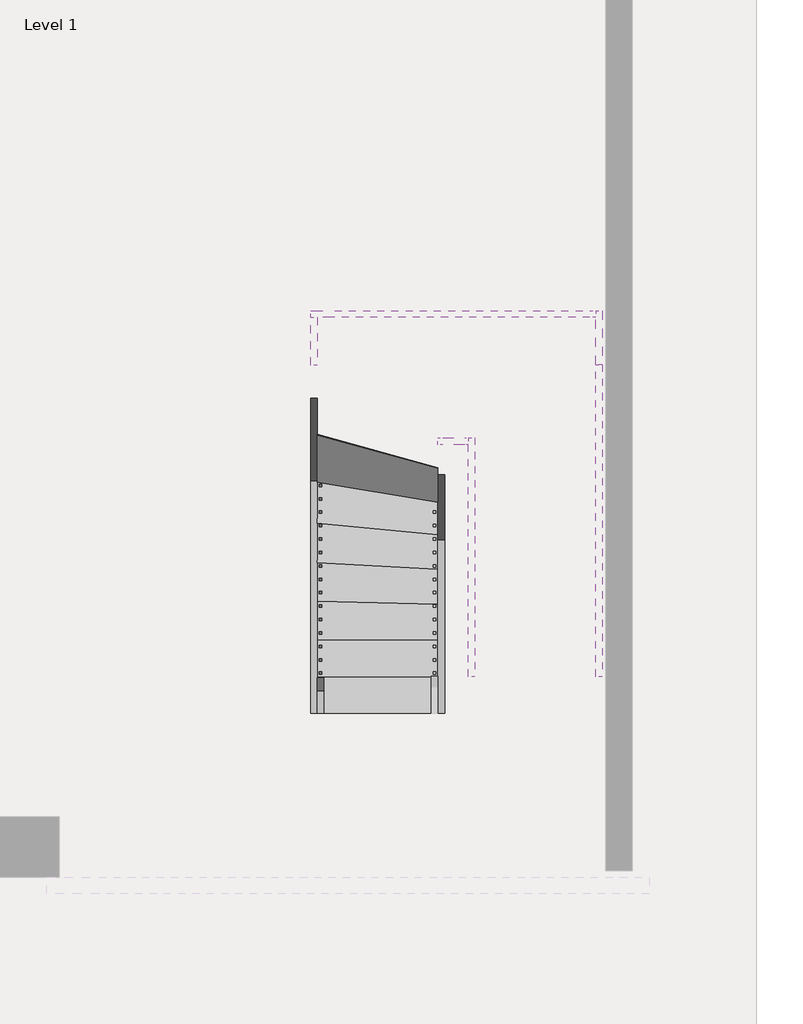
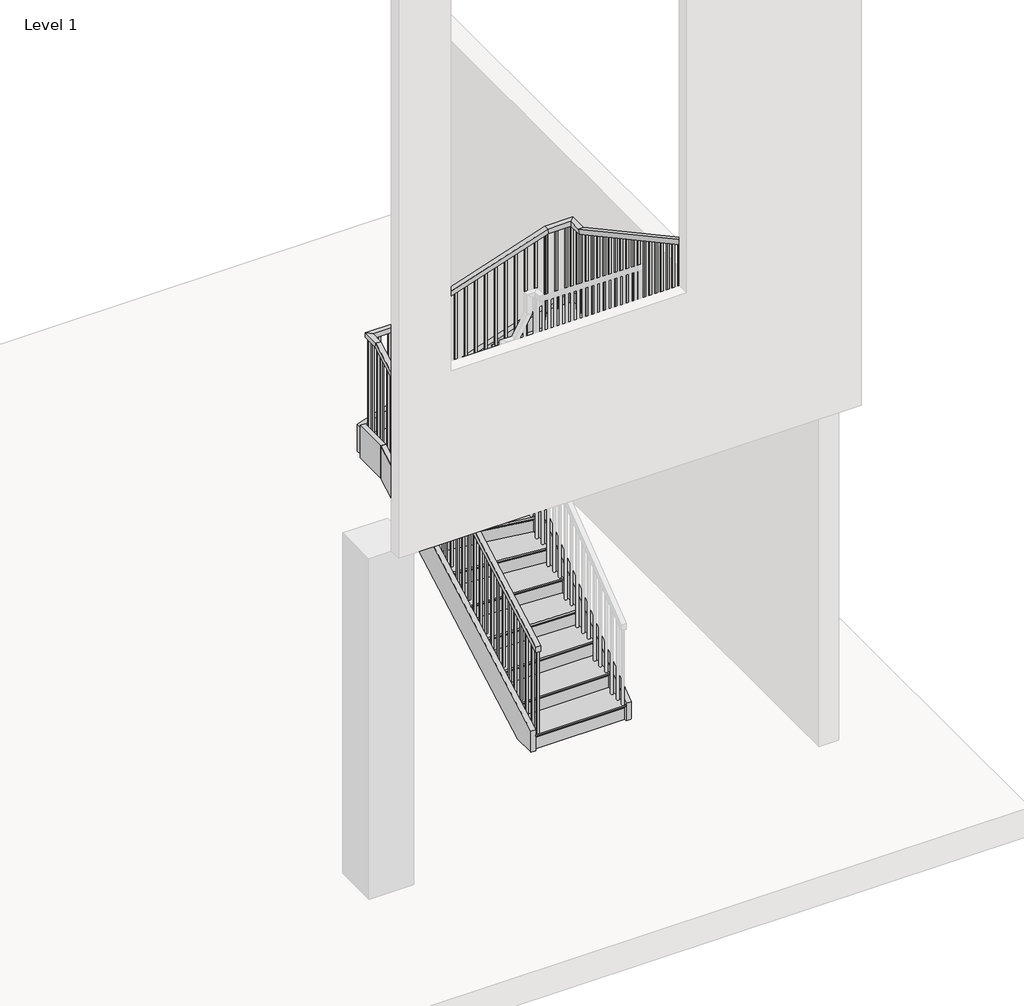
# One storey, part 2 of 2: 8 members, 1 railing, 1 stair flight.
"""IFC4 building model written with IfcOpenShell, lengths in millimetres."""

from ifc_helpers import new_model, si_unit, frame, origin, place, context, project, spatial, polyline, outline, extrude, faceted_brep, transform, mapped, element, save
from components import stair_flight_cb62f9a1

model = new_model("IFC4")

# Units and contexts
model_context = context("Model", 3, world=origin())
ifc_project = project(units=[si_unit("LENGTHUNIT", "METRE", prefix="MILLI")], contexts=[model_context])

# Site, building, storey
site = spatial("IfcSite", under=ifc_project)
building = spatial("IfcBuilding", under=site)
storey = spatial("IfcBuildingStorey", under=building, Name="Level 1", Elevation=0.0)

# Members
placement = place(None, origin())
element("IfcMember", 1, ObjectType="Stringer - 2\" Width", at=placement, inside=storey, context=model_context, shape_type="SweptSolid", body=[
    extrude(outline(polyline([(6052.3300735, 0.0), (6052.3300735, 226.8967502), (8691.4859641, 1688.3473575), (8691.4859641, 1339.9346078), (6271.7693513, 0.0), (6052.3300735, 0.0)])), frame((-8157.032922, 0.0, 0.0), z_axis=(1.0, 0.0, 0.0), x_axis=(0.0, 1.0, 0.0)), (0.0, 0.0, 1.0), 50.8),
])
element("IfcMember", 2, ObjectType="Stringer - 2\" Width", at=placement, inside=storey, context=model_context, shape_type="SweptSolid", body=[
    extrude(outline(polyline([(-8106.232922, 8691.4859641), (-8157.032922, 8691.4859641), (-8157.032922, 9053.2617654), (-8106.232922, 9053.2617654), (-8106.232922, 8691.4859641)])), frame((0.0, 0.0, 1339.9346078), z_axis=(0.0, 0.0, 1.0), x_axis=(1.0, 0.0, 0.0)), (0.0, 0.0, 1.0), 348.4127497),
])
element("IfcMember", 3, ObjectType="Stringer - 2\" Width", at=placement, inside=storey, context=model_context, shape_type="SweptSolid", body=[
    extrude(outline(polyline([(1671.581207, -8157.032922), (1383.5473575, -8157.032922), (1383.5473575, -7974.0900261), (2035.7298543, -5998.032922), (2369.5213068, -5998.032922), (2369.5213068, -6042.3341999), (1671.581207, -8157.032922)])), frame((0.0, 9053.2617654, 0.0), z_axis=(0.0, 1.0, 0.0), x_axis=(0.0, 0.0, 1.0)), (0.0, 0.0, 1.0), 50.8),
])
element("IfcMember", 4, ObjectType="Stringer - 2\" Width", at=placement, inside=storey, context=model_context, shape_type="SweptSolid", body=[
    extrude(outline(polyline([(-5998.032922, 9104.0617654), (-5947.232922, 9104.0617654), (-5947.232922, 8694.4281729), (-5998.032922, 8694.4281729), (-5998.032922, 9104.0617654)])), frame((0.0, 0.0, 2048.5496929), z_axis=(0.0, 0.0, 1.0), x_axis=(1.0, 0.0, 0.0)), (0.0, 0.0, 1.0), 320.9716139),
])
element("IfcMember", 5, ObjectType="Stringer - 2\" Width", at=placement, inside=storey, context=model_context, shape_type="SweptSolid", body=[
    extrude(outline(polyline([(8694.4281729, 2369.5213068), (8694.4281729, 2048.5496929), (6331.7300735, 3333.0016037), (6331.7300735, 3653.9732176), (8694.4281729, 2369.5213068)])), frame((-5998.032922, 0.0, 0.0), z_axis=(1.0, 0.0, 0.0), x_axis=(0.0, 1.0, 0.0)), (0.0, 0.0, 1.0), 50.8),
])
element("IfcMember", 6, ObjectType="Stringer - 2\" Width", at=placement, inside=storey, context=model_context, shape_type="SweptSolid", body=[
    extrude(outline(polyline([(6052.3300735, 0.0), (6052.3300735, 188.0018686), (8088.0617654, 1759.6054409), (8088.0617654, 1374.5429999), (6307.5868441, 0.0), (6052.3300735, 0.0)])), frame((-7191.832922, 0.0, 0.0), z_axis=(1.0, 0.0, 0.0), x_axis=(0.0, 1.0, 0.0)), (0.0, 0.0, 1.0), 50.8),
])
element("IfcMember", 7, ObjectType="Stringer - 2\" Width", at=placement, inside=storey, context=model_context, shape_type="SweptSolid", body=[
    extrude(outline(polyline([(1964.5655705, -7191.832922), (1413.7610667, -7191.832922), (1413.7610667, -7154.6813178), (1750.0370706, -6963.232922), (2320.9680273, -6963.232922), (2320.9680273, -6988.9261496), (1964.5655705, -7191.832922)])), frame((0.0, 8088.0617654, 0.0), z_axis=(0.0, 1.0, 0.0), x_axis=(0.0, 0.0, 1.0)), (0.0, 0.0, 1.0), 50.8),
])
element("IfcMember", 8, ObjectType="Stringer - 2\" Width", at=placement, inside=storey, context=model_context, shape_type="SweptSolid", body=[
    extrude(outline(polyline([(8138.8617654, 2320.9680273), (8138.8617654, 1930.7796979), (6331.7300735, 3375.0977978), (6331.7300735, 3765.2861272), (8138.8617654, 2320.9680273)])), frame((-6963.232922, 0.0, 0.0), z_axis=(1.0, 0.0, 0.0), x_axis=(0.0, 1.0, 0.0)), (0.0, 0.0, 1.0), 50.8),
])

# Railing
element("IfcRailing", 9, ObjectType="Handrail - Rectangular", at=placement, inside=storey, context=model_context, shape_type="SolidModel", body=[
    faceted_brep([(-8106.232922, 6052.3300735, 1108.0231981), (-8106.232922, 6052.3300735, 1049.9544064), (-8055.432922, 6052.3300735, 1049.9544064), (-8055.432922, 6052.3300735, 1108.0231981), (-8106.232922, 8867.2431395, 2666.8005421), (-8106.232922, 8880.3694635, 2616.0005421), (-8055.432922, 8880.3694635, 2616.0005421), (-8055.432922, 8867.2431395, 2666.8005421), (-8106.232922, 9053.2617654, 2666.8005421), (-8106.232922, 9053.2617654, 2616.0005421), (-8055.432922, 9002.4617654, 2616.0005421), (-8055.432922, 9002.4617654, 2666.8005421), (-7811.3412458, 9053.2617654, 2666.8005421), (-7803.1748117, 9053.2617654, 2616.0005421), (-7803.1748117, 9002.4617654, 2616.0005421), (-7811.3412458, 9002.4617654, 2666.8005421), (-6285.3448041, 9053.2617654, 3170.4439679), (-6277.17837, 9053.2617654, 3119.6439679), (-6277.17837, 9002.4617654, 3119.6439679), (-6285.3448041, 9002.4617654, 3170.4439679), (-5998.032922, 9053.2617654, 3170.4439679), (-5998.032922, 9053.2617654, 3119.6439679), (-6048.832922, 9002.4617654, 3119.6439679), (-6048.832922, 9002.4617654, 3170.4439679), (-5998.032922, 8868.8551356, 3170.4439679), (-5998.032922, 8855.9393392, 3119.6439679), (-6048.832922, 8855.9393392, 3119.6439679), (-6048.832922, 8868.8551356, 3170.4439679), (-5998.032922, 6331.7300735, 4549.7209626), (-6048.832922, 6331.7300735, 4549.7209626), (-6048.832922, 6331.7300735, 4491.8994479), (-5998.032922, 6331.7300735, 4491.8994479)], [[[0, 1, 2, 3]], [[1, 0, 4, 5]], [[2, 1, 5, 6]], [[3, 2, 6, 7]], [[0, 3, 7, 4]], [[5, 4, 8, 9]], [[6, 5, 9, 10]], [[7, 6, 10, 11]], [[4, 7, 11, 8]], [[9, 8, 12, 13]], [[10, 9, 13, 14]], [[11, 10, 14, 15]], [[8, 11, 15, 12]], [[13, 12, 16, 17]], [[14, 13, 17, 18]], [[15, 14, 18, 19]], [[12, 15, 19, 16]], [[17, 16, 20, 21]], [[18, 17, 21, 22]], [[19, 18, 22, 23]], [[16, 19, 23, 20]], [[21, 20, 24, 25]], [[22, 21, 25, 26]], [[23, 22, 26, 27]], [[20, 23, 27, 24]], [[28, 29, 30, 31]], [[25, 24, 28, 31]], [[26, 25, 31, 30]], [[27, 26, 30, 29]], [[24, 27, 29, 28]]]),
    extrude(outline(polyline([(6439.9801356, 4433.0506263), (6439.9801356, 3483.4285714), (6420.9301356, 3483.4285714), (6420.9301356, 4443.4069257), (6439.9801356, 4433.0506263)])), frame((-6032.957922, 0.0, 0.0), z_axis=(1.0, 0.0, 0.0), x_axis=(0.0, 1.0, 0.0)), (0.0, 0.0, 1.0), 19.05),
    extrude(outline(polyline([(6541.5801356, 4377.8170295), (6541.5801356, 3483.4285714), (6522.5301356, 3483.4285714), (6522.5301356, 4388.1733289), (6541.5801356, 4377.8170295)])), frame((-6032.957922, 0.0, 0.0), z_axis=(1.0, 0.0, 0.0), x_axis=(0.0, 1.0, 0.0)), (0.0, 0.0, 1.0), 19.05),
    extrude(outline(polyline([(6643.1801356, 4322.5834327), (6643.1801356, 3309.2571429), (6624.1301356, 3309.2571429), (6624.1301356, 4332.9397321), (6643.1801356, 4322.5834327)])), frame((-6032.957922, 0.0, 0.0), z_axis=(1.0, 0.0, 0.0), x_axis=(0.0, 1.0, 0.0)), (0.0, 0.0, 1.0), 19.05),
    extrude(outline(polyline([(6744.7801356, 4267.349836), (6744.7801356, 3309.2571429), (6725.7301356, 3309.2571429), (6725.7301356, 4277.7061354), (6744.7801356, 4267.349836)])), frame((-6032.957922, 0.0, 0.0), z_axis=(1.0, 0.0, 0.0), x_axis=(0.0, 1.0, 0.0)), (0.0, 0.0, 1.0), 19.05),
    extrude(outline(polyline([(6846.3801356, 4212.1162392), (6846.3801356, 3309.2571429), (6827.3301356, 3309.2571429), (6827.3301356, 4222.4725386), (6846.3801356, 4212.1162392)])), frame((-6032.957922, 0.0, 0.0), z_axis=(1.0, 0.0, 0.0), x_axis=(0.0, 1.0, 0.0)), (0.0, 0.0, 1.0), 19.05),
    extrude(outline(polyline([(6947.9801356, 4156.8826424), (6947.9801356, 3135.0857143), (6928.9301356, 3135.0857143), (6928.9301356, 4167.2389418), (6947.9801356, 4156.8826424)])), frame((-6032.957922, 0.0, 0.0), z_axis=(1.0, 0.0, 0.0), x_axis=(0.0, 1.0, 0.0)), (0.0, 0.0, 1.0), 19.05),
    extrude(outline(polyline([(7049.5801356, 4101.6490456), (7049.5801356, 3135.0857143), (7030.5301356, 3135.0857143), (7030.5301356, 4112.005345), (7049.5801356, 4101.6490456)])), frame((-6032.957922, 0.0, 0.0), z_axis=(1.0, 0.0, 0.0), x_axis=(0.0, 1.0, 0.0)), (0.0, 0.0, 1.0), 19.05),
    extrude(outline(polyline([(7151.1801356, 4046.4154488), (7151.1801356, 3135.0857143), (7132.1301356, 3135.0857143), (7132.1301356, 4056.7717482), (7151.1801356, 4046.4154488)])), frame((-6032.957922, 0.0, 0.0), z_axis=(1.0, 0.0, 0.0), x_axis=(0.0, 1.0, 0.0)), (0.0, 0.0, 1.0), 19.05),
    extrude(outline(polyline([(7252.7801356, 3991.1818521), (7252.7801356, 2960.9142857), (7233.7301356, 2960.9142857), (7233.7301356, 4001.5381515), (7252.7801356, 3991.1818521)])), frame((-6032.957922, 0.0, 0.0), z_axis=(1.0, 0.0, 0.0), x_axis=(0.0, 1.0, 0.0)), (0.0, 0.0, 1.0), 19.05),
    extrude(outline(polyline([(7354.3801356, 3935.9482553), (7354.3801356, 2960.9142857), (7335.3301356, 2960.9142857), (7335.3301356, 3946.3045547), (7354.3801356, 3935.9482553)])), frame((-6032.957922, 0.0, 0.0), z_axis=(1.0, 0.0, 0.0), x_axis=(0.0, 1.0, 0.0)), (0.0, 0.0, 1.0), 19.05),
    extrude(outline(polyline([(7455.9801356, 3880.7146585), (7455.9801356, 2960.9142857), (7436.9301356, 2960.9142857), (7436.9301356, 3891.0709579), (7455.9801356, 3880.7146585)])), frame((-6032.957922, 0.0, 0.0), z_axis=(1.0, 0.0, 0.0), x_axis=(0.0, 1.0, 0.0)), (0.0, 0.0, 1.0), 19.05),
    extrude(outline(polyline([(7557.5801356, 3825.4810617), (7557.5801356, 2786.7428571), (7538.5301356, 2786.7428571), (7538.5301356, 3835.8373611), (7557.5801356, 3825.4810617)])), frame((-6032.957922, 0.0, 0.0), z_axis=(1.0, 0.0, 0.0), x_axis=(0.0, 1.0, 0.0)), (0.0, 0.0, 1.0), 19.05),
    extrude(outline(polyline([(7659.1801356, 3770.2474649), (7659.1801356, 2786.7428571), (7640.1301356, 2786.7428571), (7640.1301356, 3780.6037643), (7659.1801356, 3770.2474649)])), frame((-6032.957922, 0.0, 0.0), z_axis=(1.0, 0.0, 0.0), x_axis=(0.0, 1.0, 0.0)), (0.0, 0.0, 1.0), 19.05),
    extrude(outline(polyline([(7760.7801356, 3715.0138682), (7760.7801356, 2786.7428571), (7741.7301356, 2786.7428571), (7741.7301356, 3725.3701676), (7760.7801356, 3715.0138682)])), frame((-6032.957922, 0.0, 0.0), z_axis=(1.0, 0.0, 0.0), x_axis=(0.0, 1.0, 0.0)), (0.0, 0.0, 1.0), 19.05),
    extrude(outline(polyline([(7862.3801356, 3659.7802714), (7862.3801356, 2612.5714286), (7843.3301356, 2612.5714286), (7843.3301356, 3670.1365708), (7862.3801356, 3659.7802714)])), frame((-6032.957922, 0.0, 0.0), z_axis=(1.0, 0.0, 0.0), x_axis=(0.0, 1.0, 0.0)), (0.0, 0.0, 1.0), 19.05),
    extrude(outline(polyline([(7963.9801356, 3604.5466746), (7963.9801356, 2612.5714286), (7944.9301356, 2612.5714286), (7944.9301356, 3614.902974), (7963.9801356, 3604.5466746)])), frame((-6032.957922, 0.0, 0.0), z_axis=(1.0, 0.0, 0.0), x_axis=(0.0, 1.0, 0.0)), (0.0, 0.0, 1.0), 19.05),
    extrude(outline(polyline([(8065.5801356, 3549.3130778), (8065.5801356, 2612.5714286), (8046.5301356, 2612.5714286), (8046.5301356, 3559.6693772), (8065.5801356, 3549.3130778)])), frame((-6032.957922, 0.0, 0.0), z_axis=(1.0, 0.0, 0.0), x_axis=(0.0, 1.0, 0.0)), (0.0, 0.0, 1.0), 19.05),
    extrude(outline(polyline([(8167.1801356, 3494.0794811), (8167.1801356, 2438.4), (8148.1301356, 2438.4), (8148.1301356, 3504.4357804), (8167.1801356, 3494.0794811)])), frame((-6032.957922, 0.0, 0.0), z_axis=(1.0, 0.0, 0.0), x_axis=(0.0, 1.0, 0.0)), (0.0, 0.0, 1.0), 19.05),
    extrude(outline(polyline([(8268.7801356, 3438.8458843), (8268.7801356, 2438.4), (8249.7301356, 2438.4), (8249.7301356, 3449.2021837), (8268.7801356, 3438.8458843)])), frame((-6032.957922, 0.0, 0.0), z_axis=(1.0, 0.0, 0.0), x_axis=(0.0, 1.0, 0.0)), (0.0, 0.0, 1.0), 19.05),
    extrude(outline(polyline([(8370.3801356, 3383.6122875), (8370.3801356, 2438.4), (8351.3301356, 2438.4), (8351.3301356, 3393.9685869), (8370.3801356, 3383.6122875)])), frame((-6032.957922, 0.0, 0.0), z_axis=(1.0, 0.0, 0.0), x_axis=(0.0, 1.0, 0.0)), (0.0, 0.0, 1.0), 19.05),
    extrude(outline(polyline([(8471.9801356, 3328.3786907), (8471.9801356, 2438.4), (8452.9301356, 2438.4), (8452.9301356, 3338.7349901), (8471.9801356, 3328.3786907)])), frame((-6032.957922, 0.0, 0.0), z_axis=(1.0, 0.0, 0.0), x_axis=(0.0, 1.0, 0.0)), (0.0, 0.0, 1.0), 19.05),
    extrude(outline(polyline([(8573.5801356, 3273.1450939), (8573.5801356, 2264.2285714), (8554.5301356, 2264.2285714), (8554.5301356, 3283.5013933), (8573.5801356, 3273.1450939)])), frame((-6032.957922, 0.0, 0.0), z_axis=(1.0, 0.0, 0.0), x_axis=(0.0, 1.0, 0.0)), (0.0, 0.0, 1.0), 19.05),
    extrude(outline(polyline([(8675.1801356, 3217.9114972), (8675.1801356, 2264.2285714), (8656.1301356, 2264.2285714), (8656.1301356, 3228.2677965), (8675.1801356, 3217.9114972)])), frame((-6032.957922, 0.0, 0.0), z_axis=(1.0, 0.0, 0.0), x_axis=(0.0, 1.0, 0.0)), (0.0, 0.0, 1.0), 19.05),
    extrude(outline(polyline([(8776.7801356, 3162.6779004), (8776.7801356, 2264.2285714), (8757.7301356, 2264.2285714), (8757.7301356, 3173.0341998), (8776.7801356, 3162.6779004)])), frame((-6032.957922, 0.0, 0.0), z_axis=(1.0, 0.0, 0.0), x_axis=(0.0, 1.0, 0.0)), (0.0, 0.0, 1.0), 19.05),
    extrude(outline(polyline([(-6013.907922, 8935.7867654), (-6013.907922, 8916.7367654), (-6032.957922, 8916.7367654), (-6032.957922, 8935.7867654), (-6013.907922, 8935.7867654)])), frame((0.0, 0.0, 2264.2285714), z_axis=(0.0, 0.0, 1.0), x_axis=(1.0, 0.0, 0.0)), (0.0, 0.0, 1.0), 855.4153965),
    extrude(outline(polyline([(-6091.6698041, 9037.3867654), (-6072.6198041, 9037.3867654), (-6072.6198041, 9018.3367654), (-6091.6698041, 9018.3367654), (-6091.6698041, 9037.3867654)])), frame((0.0, 0.0, 2264.2285714), z_axis=(0.0, 0.0, 1.0), x_axis=(1.0, 0.0, 0.0)), (0.0, 0.0, 1.0), 855.4153965),
    extrude(outline(polyline([(-6193.2698041, 9037.3867654), (-6174.2198041, 9037.3867654), (-6174.2198041, 9018.3367654), (-6193.2698041, 9018.3367654), (-6193.2698041, 9037.3867654)])), frame((0.0, 0.0, 2264.2285714), z_axis=(0.0, 0.0, 1.0), x_axis=(1.0, 0.0, 0.0)), (0.0, 0.0, 1.0), 855.4153965),
    extrude(outline(polyline([(3113.1461354, -6296.8662458), (2090.0571429, -6296.8662458), (2090.0571429, -6277.8162458), (3119.4334419, -6277.8162458), (3113.1461354, -6296.8662458)])), frame((0.0, 9018.3367654, 0.0), z_axis=(0.0, 1.0, 0.0), x_axis=(0.0, 0.0, 1.0)), (0.0, 0.0, 1.0), 19.05),
    extrude(outline(polyline([(3079.6138344, -6398.4662458), (2090.0571429, -6398.4662458), (2090.0571429, -6379.4162458), (3085.9011408, -6379.4162458), (3079.6138344, -6398.4662458)])), frame((0.0, 9018.3367654, 0.0), z_axis=(0.0, 1.0, 0.0), x_axis=(0.0, 0.0, 1.0)), (0.0, 0.0, 1.0), 19.05),
    extrude(outline(polyline([(3046.0815334, -6500.0662458), (2090.0571429, -6500.0662458), (2090.0571429, -6481.0162458), (3052.3688398, -6481.0162458), (3046.0815334, -6500.0662458)])), frame((0.0, 9018.3367654, 0.0), z_axis=(0.0, 1.0, 0.0), x_axis=(0.0, 0.0, 1.0)), (0.0, 0.0, 1.0), 19.05),
    extrude(outline(polyline([(3012.5492323, -6601.6662458), (2090.0571429, -6601.6662458), (2090.0571429, -6582.6162458), (3018.8365388, -6582.6162458), (3012.5492323, -6601.6662458)])), frame((0.0, 9018.3367654, 0.0), z_axis=(0.0, 1.0, 0.0), x_axis=(0.0, 0.0, 1.0)), (0.0, 0.0, 1.0), 19.05),
    extrude(outline(polyline([(2979.0169313, -6703.2662458), (2090.0571429, -6703.2662458), (2090.0571429, -6684.2162458), (2985.3042377, -6684.2162458), (2979.0169313, -6703.2662458)])), frame((0.0, 9018.3367654, 0.0), z_axis=(0.0, 1.0, 0.0), x_axis=(0.0, 0.0, 1.0)), (0.0, 0.0, 1.0), 19.05),
    extrude(outline(polyline([(2945.4846303, -6804.8662458), (2090.0571429, -6804.8662458), (2090.0571429, -6785.8162458), (2951.7719367, -6785.8162458), (2945.4846303, -6804.8662458)])), frame((0.0, 9018.3367654, 0.0), z_axis=(0.0, 1.0, 0.0), x_axis=(0.0, 0.0, 1.0)), (0.0, 0.0, 1.0), 19.05),
    extrude(outline(polyline([(2911.9523292, -6906.4662458), (1915.8857143, -6906.4662458), (1915.8857143, -6887.4162458), (2918.2396357, -6887.4162458), (2911.9523292, -6906.4662458)])), frame((0.0, 9018.3367654, 0.0), z_axis=(0.0, 1.0, 0.0), x_axis=(0.0, 0.0, 1.0)), (0.0, 0.0, 1.0), 19.05),
    extrude(outline(polyline([(2878.4200282, -7008.0662458), (1915.8857143, -7008.0662458), (1915.8857143, -6989.0162458), (2884.7073346, -6989.0162458), (2878.4200282, -7008.0662458)])), frame((0.0, 9018.3367654, 0.0), z_axis=(0.0, 1.0, 0.0), x_axis=(0.0, 0.0, 1.0)), (0.0, 0.0, 1.0), 19.05),
    extrude(outline(polyline([(2844.8877272, -7109.6662458), (1915.8857143, -7109.6662458), (1915.8857143, -7090.6162458), (2851.1750336, -7090.6162458), (2844.8877272, -7109.6662458)])), frame((0.0, 9018.3367654, 0.0), z_axis=(0.0, 1.0, 0.0), x_axis=(0.0, 0.0, 1.0)), (0.0, 0.0, 1.0), 19.05),
    extrude(outline(polyline([(2811.3554261, -7211.2662458), (1915.8857143, -7211.2662458), (1915.8857143, -7192.2162458), (2817.6427326, -7192.2162458), (2811.3554261, -7211.2662458)])), frame((0.0, 9018.3367654, 0.0), z_axis=(0.0, 1.0, 0.0), x_axis=(0.0, 0.0, 1.0)), (0.0, 0.0, 1.0), 19.05),
    extrude(outline(polyline([(2777.8231251, -7312.8662458), (1741.7142857, -7312.8662458), (1741.7142857, -7293.8162458), (2784.1104315, -7293.8162458), (2777.8231251, -7312.8662458)])), frame((0.0, 9018.3367654, 0.0), z_axis=(0.0, 1.0, 0.0), x_axis=(0.0, 0.0, 1.0)), (0.0, 0.0, 1.0), 19.05),
    extrude(outline(polyline([(2744.2908241, -7414.4662458), (1741.7142857, -7414.4662458), (1741.7142857, -7395.4162458), (2750.5781305, -7395.4162458), (2744.2908241, -7414.4662458)])), frame((0.0, 9018.3367654, 0.0), z_axis=(0.0, 1.0, 0.0), x_axis=(0.0, 0.0, 1.0)), (0.0, 0.0, 1.0), 19.05),
    extrude(outline(polyline([(2710.758523, -7516.0662458), (1741.7142857, -7516.0662458), (1741.7142857, -7497.0162458), (2717.0458295, -7497.0162458), (2710.758523, -7516.0662458)])), frame((0.0, 9018.3367654, 0.0), z_axis=(0.0, 1.0, 0.0), x_axis=(0.0, 0.0, 1.0)), (0.0, 0.0, 1.0), 19.05),
    extrude(outline(polyline([(2677.226222, -7617.6662458), (1741.7142857, -7617.6662458), (1741.7142857, -7598.6162458), (2683.5135284, -7598.6162458), (2677.226222, -7617.6662458)])), frame((0.0, 9018.3367654, 0.0), z_axis=(0.0, 1.0, 0.0), x_axis=(0.0, 0.0, 1.0)), (0.0, 0.0, 1.0), 19.05),
    extrude(outline(polyline([(2643.693921, -7719.2662458), (1741.7142857, -7719.2662458), (1741.7142857, -7700.2162458), (2649.9812274, -7700.2162458), (2643.693921, -7719.2662458)])), frame((0.0, 9018.3367654, 0.0), z_axis=(0.0, 1.0, 0.0), x_axis=(0.0, 0.0, 1.0)), (0.0, 0.0, 1.0), 19.05),
    extrude(outline(polyline([(-7887.157922, 9037.3867654), (-7868.107922, 9037.3867654), (-7868.107922, 9018.3367654), (-7887.157922, 9018.3367654), (-7887.157922, 9037.3867654)])), frame((0.0, 0.0, 1567.5428571), z_axis=(0.0, 0.0, 1.0), x_axis=(1.0, 0.0, 0.0)), (0.0, 0.0, 1.0), 1048.457685),
    extrude(outline(polyline([(-7988.757922, 9037.3867654), (-7969.707922, 9037.3867654), (-7969.707922, 9018.3367654), (-7988.757922, 9018.3367654), (-7988.757922, 9037.3867654)])), frame((0.0, 0.0, 1567.5428571), z_axis=(0.0, 0.0, 1.0), x_axis=(1.0, 0.0, 0.0)), (0.0, 0.0, 1.0), 1048.457685),
    extrude(outline(polyline([(-8090.357922, 8959.3181395), (-8090.357922, 8978.3681395), (-8071.307922, 8978.3681395), (-8071.307922, 8959.3181395), (-8090.357922, 8959.3181395)])), frame((0.0, 0.0, 1567.5428571), z_axis=(0.0, 0.0, 1.0), x_axis=(1.0, 0.0, 0.0)), (0.0, 0.0, 1.0), 1048.457685),
    extrude(outline(polyline([(8805.0550735, 2574.294684), (8805.0550735, 1567.5428571), (8786.0050735, 1567.5428571), (8786.0050735, 2563.7456164), (8805.0550735, 2574.294684)])), frame((-8090.357922, 0.0, 0.0), z_axis=(1.0, 0.0, 0.0), x_axis=(0.0, 1.0, 0.0)), (0.0, 0.0, 1.0), 19.05),
    extrude(outline(polyline([(8703.4550735, 2518.0329898), (8703.4550735, 1567.5428571), (8684.4050735, 1567.5428571), (8684.4050735, 2507.4839222), (8703.4550735, 2518.0329898)])), frame((-8090.357922, 0.0, 0.0), z_axis=(1.0, 0.0, 0.0), x_axis=(0.0, 1.0, 0.0)), (0.0, 0.0, 1.0), 19.05),
    extrude(outline(polyline([(8601.8550735, 2461.7712956), (8601.8550735, 1567.5428571), (8582.8050735, 1567.5428571), (8582.8050735, 2451.222228), (8601.8550735, 2461.7712956)])), frame((-8090.357922, 0.0, 0.0), z_axis=(1.0, 0.0, 0.0), x_axis=(0.0, 1.0, 0.0)), (0.0, 0.0, 1.0), 19.05),
    extrude(outline(polyline([(8500.2550735, 2405.5096014), (8500.2550735, 1393.3714286), (8481.2050735, 1393.3714286), (8481.2050735, 2394.9605337), (8500.2550735, 2405.5096014)])), frame((-8090.357922, 0.0, 0.0), z_axis=(1.0, 0.0, 0.0), x_axis=(0.0, 1.0, 0.0)), (0.0, 0.0, 1.0), 19.05),
    extrude(outline(polyline([(8398.6550735, 2349.2479072), (8398.6550735, 1393.3714286), (8379.6050735, 1393.3714286), (8379.6050735, 2338.6988395), (8398.6550735, 2349.2479072)])), frame((-8090.357922, 0.0, 0.0), z_axis=(1.0, 0.0, 0.0), x_axis=(0.0, 1.0, 0.0)), (0.0, 0.0, 1.0), 19.05),
    extrude(outline(polyline([(8297.0550735, 2292.986213), (8297.0550735, 1393.3714286), (8278.0050735, 1393.3714286), (8278.0050735, 2282.4371453), (8297.0550735, 2292.986213)])), frame((-8090.357922, 0.0, 0.0), z_axis=(1.0, 0.0, 0.0), x_axis=(0.0, 1.0, 0.0)), (0.0, 0.0, 1.0), 19.05),
    extrude(outline(polyline([(8195.4550735, 2236.7245188), (8195.4550735, 1393.3714286), (8176.4050735, 1393.3714286), (8176.4050735, 2226.1754511), (8195.4550735, 2236.7245188)])), frame((-8090.357922, 0.0, 0.0), z_axis=(1.0, 0.0, 0.0), x_axis=(0.0, 1.0, 0.0)), (0.0, 0.0, 1.0), 19.05),
    extrude(outline(polyline([(8093.8550735, 2180.4628245), (8093.8550735, 1219.2), (8074.8050735, 1219.2), (8074.8050735, 2169.9137569), (8093.8550735, 2180.4628245)])), frame((-8090.357922, 0.0, 0.0), z_axis=(1.0, 0.0, 0.0), x_axis=(0.0, 1.0, 0.0)), (0.0, 0.0, 1.0), 19.05),
    extrude(outline(polyline([(7992.2550735, 2124.2011303), (7992.2550735, 1219.2), (7973.2050735, 1219.2), (7973.2050735, 2113.6520627), (7992.2550735, 2124.2011303)])), frame((-8090.357922, 0.0, 0.0), z_axis=(1.0, 0.0, 0.0), x_axis=(0.0, 1.0, 0.0)), (0.0, 0.0, 1.0), 19.05),
    extrude(outline(polyline([(7890.6550735, 2067.9394361), (7890.6550735, 1219.2), (7871.6050735, 1219.2), (7871.6050735, 2057.3903685), (7890.6550735, 2067.9394361)])), frame((-8090.357922, 0.0, 0.0), z_axis=(1.0, 0.0, 0.0), x_axis=(0.0, 1.0, 0.0)), (0.0, 0.0, 1.0), 19.05),
    extrude(outline(polyline([(7789.0550735, 2011.6777419), (7789.0550735, 1045.0285714), (7770.0050735, 1045.0285714), (7770.0050735, 2001.1286742), (7789.0550735, 2011.6777419)])), frame((-8090.357922, 0.0, 0.0), z_axis=(1.0, 0.0, 0.0), x_axis=(0.0, 1.0, 0.0)), (0.0, 0.0, 1.0), 19.05),
    extrude(outline(polyline([(7687.4550735, 1955.4160477), (7687.4550735, 1045.0285714), (7668.4050735, 1045.0285714), (7668.4050735, 1944.86698), (7687.4550735, 1955.4160477)])), frame((-8090.357922, 0.0, 0.0), z_axis=(1.0, 0.0, 0.0), x_axis=(0.0, 1.0, 0.0)), (0.0, 0.0, 1.0), 19.05),
    extrude(outline(polyline([(7585.8550735, 1899.1543535), (7585.8550735, 1045.0285714), (7566.8050735, 1045.0285714), (7566.8050735, 1888.6052858), (7585.8550735, 1899.1543535)])), frame((-8090.357922, 0.0, 0.0), z_axis=(1.0, 0.0, 0.0), x_axis=(0.0, 1.0, 0.0)), (0.0, 0.0, 1.0), 19.05),
    extrude(outline(polyline([(7484.2550735, 1842.8926593), (7484.2550735, 870.8571429), (7465.2050735, 870.8571429), (7465.2050735, 1832.3435916), (7484.2550735, 1842.8926593)])), frame((-8090.357922, 0.0, 0.0), z_axis=(1.0, 0.0, 0.0), x_axis=(0.0, 1.0, 0.0)), (0.0, 0.0, 1.0), 19.05),
    extrude(outline(polyline([(7382.6550735, 1786.6309651), (7382.6550735, 870.8571429), (7363.6050735, 870.8571429), (7363.6050735, 1776.0818974), (7382.6550735, 1786.6309651)])), frame((-8090.357922, 0.0, 0.0), z_axis=(1.0, 0.0, 0.0), x_axis=(0.0, 1.0, 0.0)), (0.0, 0.0, 1.0), 19.05),
    extrude(outline(polyline([(7281.0550735, 1730.3692708), (7281.0550735, 870.8571429), (7262.0050735, 870.8571429), (7262.0050735, 1719.8202032), (7281.0550735, 1730.3692708)])), frame((-8090.357922, 0.0, 0.0), z_axis=(1.0, 0.0, 0.0), x_axis=(0.0, 1.0, 0.0)), (0.0, 0.0, 1.0), 19.05),
    extrude(outline(polyline([(7179.4550735, 1674.1075766), (7179.4550735, 696.6857143), (7160.4050735, 696.6857143), (7160.4050735, 1663.558509), (7179.4550735, 1674.1075766)])), frame((-8090.357922, 0.0, 0.0), z_axis=(1.0, 0.0, 0.0), x_axis=(0.0, 1.0, 0.0)), (0.0, 0.0, 1.0), 19.05),
    extrude(outline(polyline([(7077.8550735, 1617.8458824), (7077.8550735, 696.6857143), (7058.8050735, 696.6857143), (7058.8050735, 1607.2968147), (7077.8550735, 1617.8458824)])), frame((-8090.357922, 0.0, 0.0), z_axis=(1.0, 0.0, 0.0), x_axis=(0.0, 1.0, 0.0)), (0.0, 0.0, 1.0), 19.05),
    extrude(outline(polyline([(6976.2550735, 1561.5841882), (6976.2550735, 696.6857143), (6957.2050735, 696.6857143), (6957.2050735, 1551.0351205), (6976.2550735, 1561.5841882)])), frame((-8090.357922, 0.0, 0.0), z_axis=(1.0, 0.0, 0.0), x_axis=(0.0, 1.0, 0.0)), (0.0, 0.0, 1.0), 19.05),
    extrude(outline(polyline([(6874.6550735, 1505.322494), (6874.6550735, 522.5142857), (6855.6050735, 522.5142857), (6855.6050735, 1494.7734263), (6874.6550735, 1505.322494)])), frame((-8090.357922, 0.0, 0.0), z_axis=(1.0, 0.0, 0.0), x_axis=(0.0, 1.0, 0.0)), (0.0, 0.0, 1.0), 19.05),
    extrude(outline(polyline([(6773.0550735, 1449.0607998), (6773.0550735, 522.5142857), (6754.0050735, 522.5142857), (6754.0050735, 1438.5117321), (6773.0550735, 1449.0607998)])), frame((-8090.357922, 0.0, 0.0), z_axis=(1.0, 0.0, 0.0), x_axis=(0.0, 1.0, 0.0)), (0.0, 0.0, 1.0), 19.05),
    extrude(outline(polyline([(6671.4550735, 1392.7991056), (6671.4550735, 522.5142857), (6652.4050735, 522.5142857), (6652.4050735, 1382.2500379), (6671.4550735, 1392.7991056)])), frame((-8090.357922, 0.0, 0.0), z_axis=(1.0, 0.0, 0.0), x_axis=(0.0, 1.0, 0.0)), (0.0, 0.0, 1.0), 19.05),
    extrude(outline(polyline([(6569.8550735, 1336.5374113), (6569.8550735, 348.3428571), (6550.8050735, 348.3428571), (6550.8050735, 1325.9883437), (6569.8550735, 1336.5374113)])), frame((-8090.357922, 0.0, 0.0), z_axis=(1.0, 0.0, 0.0), x_axis=(0.0, 1.0, 0.0)), (0.0, 0.0, 1.0), 19.05),
    extrude(outline(polyline([(6468.2550735, 1280.2757171), (6468.2550735, 348.3428571), (6449.2050735, 348.3428571), (6449.2050735, 1269.7266495), (6468.2550735, 1280.2757171)])), frame((-8090.357922, 0.0, 0.0), z_axis=(1.0, 0.0, 0.0), x_axis=(0.0, 1.0, 0.0)), (0.0, 0.0, 1.0), 19.05),
    extrude(outline(polyline([(6366.6550735, 1224.0140229), (6366.6550735, 348.3428571), (6347.6050735, 348.3428571), (6347.6050735, 1213.4649553), (6366.6550735, 1224.0140229)])), frame((-8090.357922, 0.0, 0.0), z_axis=(1.0, 0.0, 0.0), x_axis=(0.0, 1.0, 0.0)), (0.0, 0.0, 1.0), 19.05),
    extrude(outline(polyline([(6265.0550735, 1167.7523287), (6265.0550735, 174.1714286), (6246.0050735, 174.1714286), (6246.0050735, 1157.203261), (6265.0550735, 1167.7523287)])), frame((-8090.357922, 0.0, 0.0), z_axis=(1.0, 0.0, 0.0), x_axis=(0.0, 1.0, 0.0)), (0.0, 0.0, 1.0), 19.05),
    extrude(outline(polyline([(6163.4550735, 1111.4906345), (6163.4550735, 174.1714286), (6144.4050735, 174.1714286), (6144.4050735, 1100.9415668), (6163.4550735, 1111.4906345)])), frame((-8090.357922, 0.0, 0.0), z_axis=(1.0, 0.0, 0.0), x_axis=(0.0, 1.0, 0.0)), (0.0, 0.0, 1.0), 19.05),
    extrude(outline(polyline([(-6013.907922, 8878.3801356), (-6013.907922, 8859.3301356), (-6032.957922, 8859.3301356), (-6032.957922, 8878.3801356), (-6013.907922, 8878.3801356)])), frame((0.0, 0.0, 2264.2285714), z_axis=(0.0, 0.0, 1.0), x_axis=(1.0, 0.0, 0.0)), (0.0, 0.0, 1.0), 855.4153965),
    extrude(outline(polyline([(-6032.957922, 9037.3867654), (-6013.907922, 9037.3867654), (-6013.907922, 9018.3367654), (-6032.957922, 9018.3367654), (-6032.957922, 9037.3867654)])), frame((0.0, 0.0, 2264.2285714), z_axis=(0.0, 0.0, 1.0), x_axis=(1.0, 0.0, 0.0)), (0.0, 0.0, 1.0), 855.4153965),
    extrude(outline(polyline([(3113.8050457, -6294.8698041), (2090.0571429, -6294.8698041), (2090.0571429, -6275.8198041), (3120.0923522, -6275.8198041), (3113.8050457, -6294.8698041)])), frame((0.0, 9018.3367654, 0.0), z_axis=(0.0, 1.0, 0.0), x_axis=(0.0, 0.0, 1.0)), (0.0, 0.0, 1.0), 19.05),
    extrude(outline(polyline([(-7820.8662458, 9037.3867654), (-7801.8162458, 9037.3867654), (-7801.8162458, 9018.3367654), (-7820.8662458, 9018.3367654), (-7820.8662458, 9037.3867654)])), frame((0.0, 0.0, 1741.7142857), z_axis=(0.0, 0.0, 1.0), x_axis=(1.0, 0.0, 0.0)), (0.0, 0.0, 1.0), 874.2862564),
    extrude(outline(polyline([(-8090.357922, 9018.3367654), (-8090.357922, 9037.3867654), (-8071.307922, 9037.3867654), (-8071.307922, 9018.3367654), (-8090.357922, 9018.3367654)])), frame((0.0, 0.0, 1567.5428571), z_axis=(0.0, 0.0, 1.0), x_axis=(1.0, 0.0, 0.0)), (0.0, 0.0, 1.0), 1048.457685),
    extrude(outline(polyline([(8876.7681395, 2614.0062844), (8876.7681395, 1567.5428571), (8857.7181395, 1567.5428571), (8857.7181395, 2603.4572167), (8876.7681395, 2614.0062844)])), frame((-8090.357922, 0.0, 0.0), z_axis=(1.0, 0.0, 0.0), x_axis=(0.0, 1.0, 0.0)), (0.0, 0.0, 1.0), 19.05),
    extrude(outline(polyline([(6350.7800735, 4481.5431486), (6350.7800735, 3483.4285714), (6331.7300735, 3483.4285714), (6331.7300735, 4491.8994479), (6350.7800735, 4481.5431486)])), frame((-6032.957922, 0.0, 0.0), z_axis=(1.0, 0.0, 0.0), x_axis=(0.0, 1.0, 0.0)), (0.0, 0.0, 1.0), 19.05),
    extrude(outline(polyline([(6071.3800735, 1060.5034741), (6071.3800735, 174.1714286), (6052.3300735, 174.1714286), (6052.3300735, 1049.9544064), (6071.3800735, 1060.5034741)])), frame((-8090.357922, 0.0, 0.0), z_axis=(1.0, 0.0, 0.0), x_axis=(0.0, 1.0, 0.0)), (0.0, 0.0, 1.0), 19.05),
])

# Stair flight
stair_flight_shape = stair_flight_cb62f9a1(model_context)
element("IfcStairFlight", 10, ObjectType="2\" Tread 1\" Nosing 1/4\" Riser", at=placement, inside=storey, context=model_context, shape_type="MappedRepresentation", body=[
    mapped(stair_flight_shape, transform((0.0, 0.0, 0.0), x_axis=(1.0, 0.0, 0.0), y_axis=(0.0, 1.0, 0.0), z_axis=(0.0, 0.0, 1.0))),
])

save(model, "model.ifc")

# Revit data of these elements
# Type "Handrail - Rectangular"
#   Assembly Code = "C2010400"
#   built-in parameter 1008612 = 0.0416667 (stored number, unit not read)
#   built-in parameter 1008611 = 0.0416667 (stored number, unit not read)
#   built-in parameter 1008609 = 0.333333 (stored number, unit not read)
#   built-in parameter 1008604 = 0.166667 (stored number, unit not read)
#   built-in parameter 1008603 = 0.166667 (stored number, unit not read)
#   Railing Height = 3' - 0"
#   built-in parameter 1008630 = 2
#   built-in parameter 1008610 = 2
#   built-in parameter 1008618 = Baluster - Square : 3/4"
# Elements 1, 2, 3, 4, 5, 6, 7, 8 (IfcMember, "Stringer - 2\" Width")
#   Phase Created = New Construction
# Element 9 (IfcRailing, "Handrail - Rectangular")
#   Phase Created = New Construction
# Element 10 (IfcStairFlight, "2\" Tread 1\" Nosing 1/4\" Riser")
#   Phase Created = New Construction
